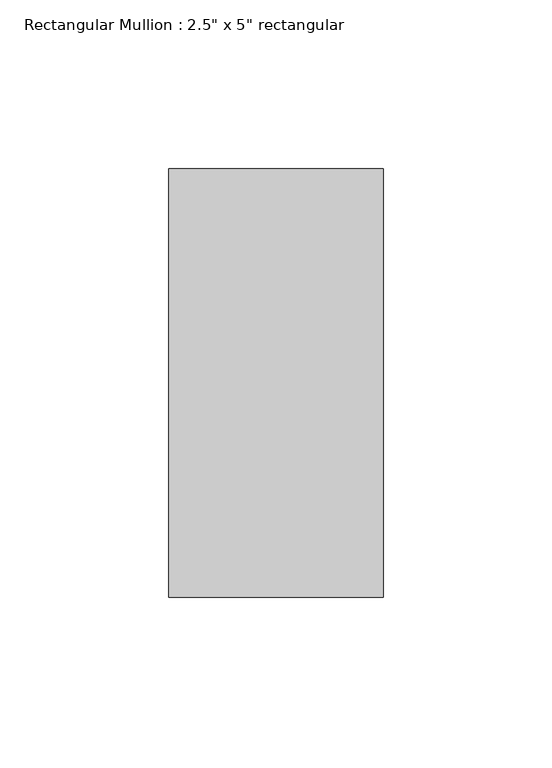
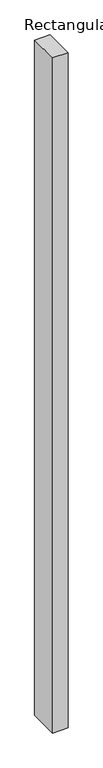
"""IFC4 building model written with IfcOpenShell, lengths in millimetres: member geometry."""

from ifc_helpers import new_model, si_unit, frame, origin, place, context, project, spatial, polyline, outline, extrude, source, transform, mapped, element, save


def member_d457d5cf(model_context):
    return source(origin(), model_context, "Body", "SweptSolid", [
        extrude(outline(polyline([(0.0, 63.5), (0.0, -63.5), (-63.5, -63.5), (-63.5, 63.5), (0.0, 63.5)])), frame((0.0, 0.0, -2921.0), z_axis=(0.0, 0.0, 1.0), x_axis=(1.0, 0.0, 0.0)), (0.0, 0.0, 1.0), 2921.0),
    ])


if __name__ == "__main__":
    model = new_model("IFC4")
    model_context = context("Model", 3, world=origin())
    ifc_project = project(units=[si_unit("LENGTHUNIT", "METRE", prefix="MILLI")], contexts=[model_context])
    site = spatial("IfcSite", under=ifc_project)
    building = spatial("IfcBuilding", under=site)
    placement = place(None, origin())
    member_shape = member_d457d5cf(model_context)
    element("IfcMember", 1, ObjectType="Rectangular Mullion : 2.5\" x 5\" rectangular", at=placement, inside=building, context=model_context, shape_type="MappedRepresentation", body=[
        mapped(member_shape, transform((0.0, 0.0, 0.0), x_axis=(1.0, 0.0, 0.0), y_axis=(0.0, 1.0, 0.0), z_axis=(0.0, 0.0, 1.0))),
    ])
    save(model, "model.ifc")

# Revit data of these elements
# Type "Rectangular Mullion : 2.5\" x 5\" rectangular"
#   built-in parameter 1007304 = 0.416667 (stored number, unit not read)
#   built-in parameter 1007301 = 0.104167 (stored number, unit not read)
#   built-in parameter 1007300 = 0.104167 (stored number, unit not read)
# Element 1 (IfcMember, "Rectangular Mullion : 2.5\" x 5\" rectangular")
#   Materials on its faces: "Iron, Ductile"
# Materials
#   "Iron, Ductile": class "Metal", colour RGB 0 0 0, transparency 0, Description = "Ductile cast iron", Cost = 0
